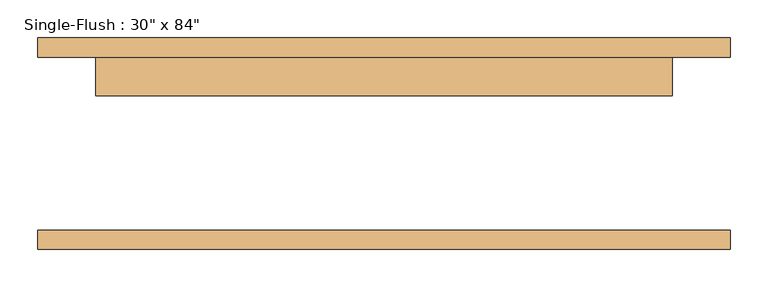
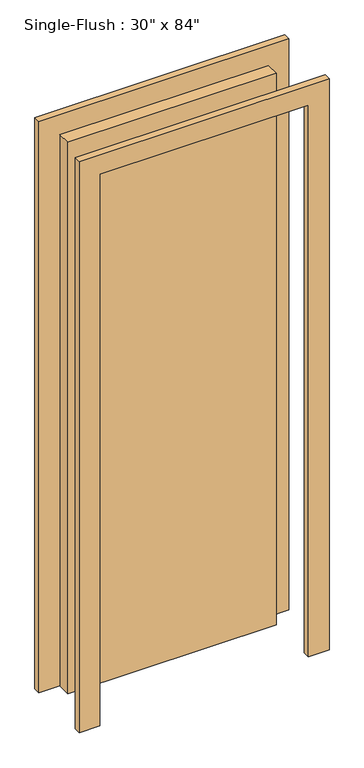
"""IFC4 building model written with IfcOpenShell, lengths in millimetres: door geometry."""

from ifc_helpers import new_model, si_unit, frame, origin, origin_with_axes, place, context, project, spatial, polyline, outline, extrude, source, transform, mapped, element, save


def door_bb98abfd(model_context):
    return source(origin(), model_context, "Body", "SweptSolid", [
        extrude(outline(polyline([(2209.8, -457.2), (0.0, -457.2), (0.0, -381.0), (2133.6, -381.0), (2133.6, 381.0), (0.0, 381.0), (0.0, 457.2), (2209.8, 457.2), (2209.8, -457.2)])), frame((0.0, 114.3, 0.0), z_axis=(0.0, 1.0, 0.0), x_axis=(0.0, 0.0, 1.0)), (0.0, 0.0, 1.0), 25.4),
        extrude(outline(polyline([(2209.8, 457.2), (2209.8, -457.2), (0.0, -457.2), (0.0, -381.0), (2133.6, -381.0), (2133.6, 381.0), (0.0, 381.0), (0.0, 457.2), (2209.8, 457.2)])), frame((0.0, -139.7, 0.0), z_axis=(0.0, 1.0, 0.0), x_axis=(0.0, 0.0, 1.0)), (0.0, 0.0, 1.0), 25.4),
        extrude(outline(polyline([(381.0, 63.5), (-381.0, 63.5), (-381.0, 114.3), (381.0, 114.3), (381.0, 63.5)])), origin_with_axes(), (0.0, 0.0, 1.0), 2133.6),
    ])


if __name__ == "__main__":
    model = new_model("IFC4")
    model_context = context("Model", 3, world=origin())
    ifc_project = project(units=[si_unit("LENGTHUNIT", "METRE", prefix="MILLI")], contexts=[model_context])
    site = spatial("IfcSite", under=ifc_project)
    building = spatial("IfcBuilding", under=site)
    placement = place(None, origin())
    door_shape = door_bb98abfd(model_context)
    element("IfcDoor", 1, ObjectType="Single-Flush : 30\" x 84\"", at=placement, inside=building, context=model_context, shape_type="MappedRepresentation", body=[
        mapped(door_shape, transform((0.0, 0.0, 0.0), x_axis=(1.0, 0.0, 0.0), y_axis=(0.0, 1.0, 0.0), z_axis=(0.0, 0.0, 1.0))),
    ])
    save(model, "model.ifc")

# Revit data of these elements
# Type "Single-Flush : 30\" x 84\""
#   Type Mark = "4"
#   Construction Type Id = "MDOOR"
#   Assembly Code = "C1020"
#   Analytic Construction = "Metal"
#   Thickness = 0' - 2"
#   Heat Transfer Coefficient (U) = 0.651978 BTU/(h·ft²·°F)
#   Height = 7' - 0"
#   Trim Projection Ext = 0' - 1"
#   Trim Projection Int = 0' - 1"
#   Trim Width = 0' - 3"
#   Width = 2' - 6"
#   Define Thermal Properties by = 1
#   Door Material = Door - Panel
#   Frame Material = Door - Frame
#   Visual Light Transmittance = 0
#   Solar Heat Gain Coefficient = 0
#   Function = (empty or 0)
#   Wall Closure = (empty or 0)
# Element 1 (IfcDoor, "Single-Flush : 30\" x 84\"")
#   Materials on its faces: "Door - Frame", "Door - Panel"
# Materials
#   "Door - Panel": class "Wood", colour RGB 210 159 95, transparency 0
#   "Door - Frame": colour RGB 118 70 51, transparency 0
